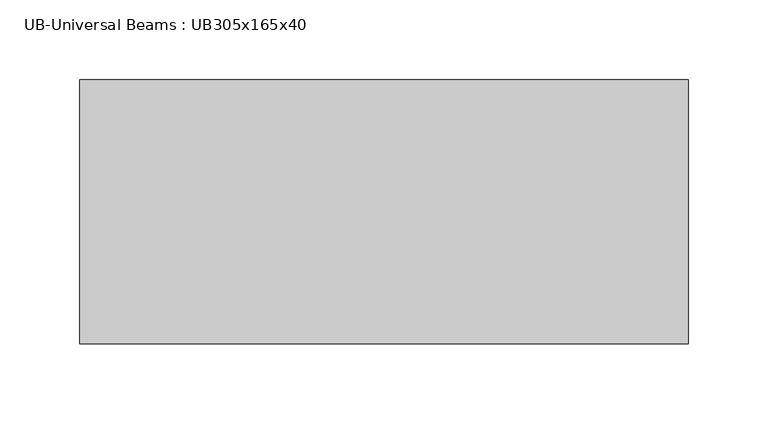
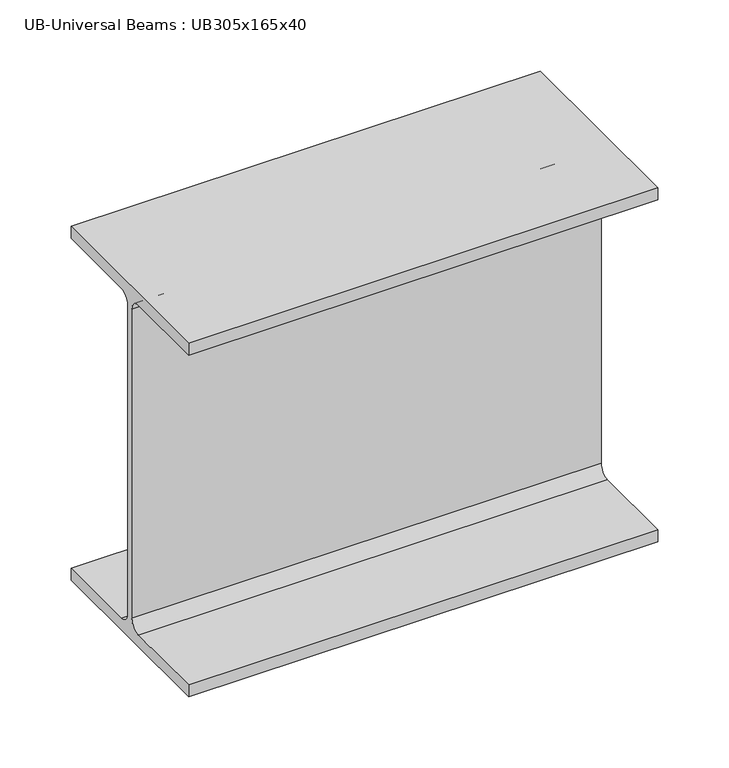
"""IFC4 building model written with IfcOpenShell, lengths in millimetres: beam geometry, UB-Universal Beams : UB305x165x40."""

from ifc_helpers import new_model, si_unit, point, frame, frame_2d, origin, place, context, project, spatial, polyline, circle_curve, trimmed, segment, composite_curve, outline, extrude, source, transform, mapped, element, save


def ub_universal_beams_ub305x165x40_491b1046(model_context):
    return source(origin(), model_context, "Body", "SweptSolid", [
        extrude(outline(composite_curve([segment(polyline([(-82.5, -141.5), (-11.9, -141.5)]), True, "CONTINUOUS"), segment(trimmed(circle_curve(frame_2d((-11.9, -132.6)), 8.9), [point((-11.9, -141.5))], [point((-3.0, -132.6))], True, "CARTESIAN"), True, "CONTINUOUS"), segment(polyline([(-3.0, -132.6), (-3.0, 132.6)]), True, "CONTINUOUS"), segment(trimmed(circle_curve(frame_2d((-11.9, 132.6)), 8.9), [point((-3.0, 132.6))], [point((-11.9, 141.5))], True, "CARTESIAN"), True, "CONTINUOUS"), segment(polyline([(-11.9, 141.5), (-82.5, 141.5), (-82.5, 151.7), (82.5, 151.7), (82.5, 141.5), (11.9, 141.5)]), True, "CONTINUOUS"), segment(trimmed(circle_curve(frame_2d((11.9, 132.6)), 8.9), [point((11.9, 141.5))], [point((3.0, 132.6))], True, "CARTESIAN"), True, "CONTINUOUS"), segment(polyline([(3.0, 132.6), (3.0, -132.6)]), True, "CONTINUOUS"), segment(trimmed(circle_curve(frame_2d((11.9, -132.6)), 8.9), [point((3.0, -132.6))], [point((11.9, -141.5))], True, "CARTESIAN"), True, "CONTINUOUS"), segment(polyline([(11.9, -141.5), (82.5, -141.5), (82.5, -151.7), (-82.5, -151.7), (-82.5, -141.5)]), True, "CONTINUOUS")], self_intersect=False)), frame((415.75, 0.0, 0.0), z_axis=(1.0, 0.0, 0.0), x_axis=(0.0, 1.0, 0.0)), (0.0, 0.0, 1.0), 380.6),
    ])


if __name__ == "__main__":
    model = new_model("IFC4")
    model_context = context("Model", 3, world=origin())
    ifc_project = project(units=[si_unit("LENGTHUNIT", "METRE", prefix="MILLI")], contexts=[model_context])
    site = spatial("IfcSite", under=ifc_project)
    building = spatial("IfcBuilding", under=site)
    placement = place(None, origin())
    ub_universal_beams_ub305x165x40_shape = ub_universal_beams_ub305x165x40_491b1046(model_context)
    element("IfcBeam", 1, ObjectType="UB-Universal Beams : UB305x165x40", at=placement, inside=building, context=model_context, shape_type="MappedRepresentation", body=[
        mapped(ub_universal_beams_ub305x165x40_shape, transform((0.0, 0.0, 0.0), x_axis=(1.0, 0.0, 0.0), y_axis=(0.0, 1.0, 0.0), z_axis=(0.0, 0.0, 1.0))),
    ])
    save(model, "model.ifc")

# Revit data of these elements
# Type "UB-Universal Beams : UB305x165x40"
#   Section Name Key = "UB305X165X40"
#   Width = 16.5 cm
#   Web Thickness = 0.6 cm
#   Web Fillet = 0.89 cm
#   Warping Constant = 164000.0 cm⁶
#   Torsional Moment of Inertia = 14.70 cm⁴
#   Section Area = 51.3 cm²
#   Plastic Modulus weak axis = 142.0 cm³
#   Plastic Modulus strong axis = 623.0 cm³
#   Nominal Weight = 40.2999 kgf/m
#   Moment of Inertia weak axis = 764.00 cm⁴
#   Moment of Inertia strong axis = 8503.00 cm⁴
#   Height = 30.34 cm
#   Flange Thickness = 1.02 cm
#   Elastic Modulus weak axis = 92.6 cm³
#   Elastic Modulus strong axis = 560.0 cm³
#   Centroid Vertical = 15.17 cm
#   Centroid Horizontal = 8.25 cm
#   Bolt Spacing = 9.0 cm
#   Length [instance default] = 1500 mm
#   Structural Material [instance default] = Metal - Steel 43-275
#   Type Comments = ""
#   Assembly Code = ""
# Element 1 (IfcBeam, "UB-Universal Beams : UB305x165x40")
#   Materials on its faces: "Metal - Steel 43-275"
# Materials
#   "Metal - Steel 43-275": class "Metal", colour RGB 247 247 247, transparency 0, Cost = 0
